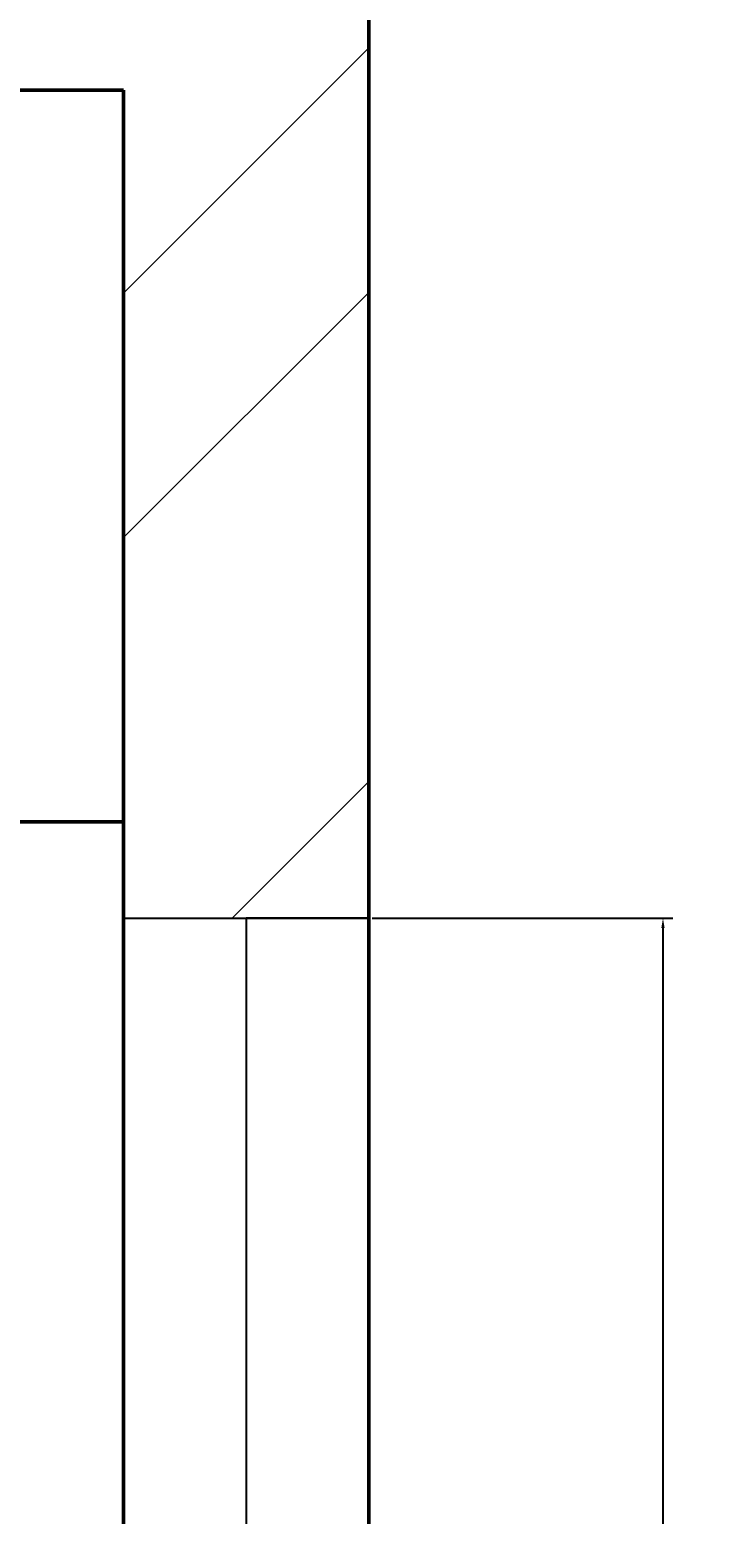
# Model space of a CAD drawing. Units: inches. Extents: x 1901 to 2863, y 888 to 2433.
# Tile 89 of 91: x 2747 to 2759, y 2052 to 2080. Entities that reach past the tile are written whole.
import ezdxf

# ---------------------------------------------------------------- set-up
doc = ezdxf.new("R2010")
doc.units = ezdxf.units.IN
for name, color, linetype, lineweight in [('A-ANNO-DIMS', 2, 'Continuous', 18), ('A-GLAZ', 3, 'Continuous', 25), ('A-WALL', 7, 'Continuous', 50), ('A-WALL-PATT', 8, 'Continuous', 13)]:
    doc.layers.add(name, color=color, linetype=linetype, lineweight=lineweight)
doc.styles.get("Standard").update_dxf_attribs({"font": 'arial.ttf'})
doc.dimstyles.get("Standard").update_dxf_attribs({"dimtxt": 0.18, "dimasz": 0.18, "dimexe": 0.18, "dimexo": 0.0625, "dimgap": 0.09, "dimtad": 0, "dimtih": 1, "dimtoh": 1, "dimdec": 4, "dimzin": 0, "dimdsep": 46, "dimtxsty": 'Standard', "dimcen": 0.09, "dimadec": 0, "dimazin": 0, "dimtfac": 1, "dimtdec": 4, "dimtofl": 0, "dimtmove": 0, "dimatfit": 3, "dimfxl": 1, "dimtolj": 1, "dimtzin": 0, "dimarcsym": 0})

# ---------------------------------------------------------------- blocks, each defined once
blk = doc.blocks.new('WIN-36-5')
for p, q in [((0, 36), (4.5, 36)), ((4.5, 36), (2.25, 36)), ((2.25, 36), (2.25, 0))]:
    blk.add_line(p, q)
blk = doc.blocks.new('*D29')
at = {"layer": 'A-ANNO-DIMS', "color": 0, "lineweight": -2, "transparency": 16777216}
for p, q in [((2752.989, 2063.429), (2758.506, 2063.429)), ((2758.326, 2063.249), (2758.326, 2045.612)), ((2758.326, 2027.609), (2758.326, 2045.245)), ((2752.989, 2027.429), (2758.506, 2027.429))]:
    blk.add_line(p, q, dxfattribs=at)
at = {"layer": 'A-ANNO-DIMS', "color": 0, "transparency": 16777216}
for points in [[(2758.296, 2063.249), (2758.356, 2063.249), (2758.326, 2063.429)], [(2758.296, 2027.609), (2758.356, 2027.609), (2758.326, 2027.429)]]:
    blk.add_solid(points, dxfattribs=at)
at = {"layer": 'Defpoints', "color": 0, "transparency": 16777216}
for p in [(2752.926, 2063.429), (2758.326, 2063.429), (2752.926, 2027.429)]:
    blk.add_point(p, dxfattribs=at)
at = {"layer": 'A-ANNO-DIMS', "color": 0, "transparency": 16777216, "insert": (2758.326, 2045.429), "char_height": 0.18, "attachment_point": 5}
blk.add_mtext('\\A1;WINDOW W6 36 TYP.', dxfattribs=at)

msp = doc.modelspace()

# ---------------------------------------------------------------- hatches: boundary and pattern name
at = {"layer": 'A-WALL-PATT'}
h = msp.add_hatch(dxfattribs=at)
h.set_pattern_fill('ANSI32', color=256)
h.paths.add_polyline_path([(2192.501, 2274.134), (2141.264, 2274.134), (2141.264, 2269.634), (2192.501, 2269.634)])
h.paths.add_polyline_path([(2259.926, 2274.134), (2216.501, 2274.134), (2216.501, 2269.634), (2255.426, 2269.634), (2255.426, 2214.634), (2250.809, 2214.634), (2250.809, 2210.134), (2259.926, 2210.134), (2259.926, 2215.134), (2271.756, 2215.134), (2271.756, 2217.384), (2271.756, 2219.634), (2259.926, 2219.634)])
h.paths.add_polyline_path([(2171.426, 2269.634), (2166.926, 2269.634), (2166.926, 2219.634), (2121.238, 2219.634), (2121.238, 2215.134), (2166.926, 2215.134), (2166.926, 2083.134), (2161.807, 2083.134), (2161.807, 2078.634), (2171.426, 2078.634), (2176.996, 2078.634), (2176.996, 2080.884), (2176.996, 2083.134), (2171.426, 2083.134), (2171.426, 2210.134), (2230.912, 2210.134), (2230.912, 2212.384), (2230.912, 2214.634), (2171.426, 2214.634)])
h.paths.add_polyline_path([(2117.264, 2274.134), (2089.426, 2274.134), (2089.426, 2219.634), (2081.136, 2219.634), (2081.136, 2215.134), (2089.426, 2215.134), (2098.004, 2215.134), (2098.004, 2217.384), (2098.004, 2219.634), (2093.926, 2219.634), (2093.926, 2269.634), (2117.264, 2269.634), (2117.264, 2271.884)])
h.paths.add_polyline_path([(2343.426, 2219.634), (2329.295, 2219.634), (2329.295, 2215.134), (2338.926, 2215.134), (2338.926, 2184.739), (2343.426, 2184.739)])
h.paths.add_polyline_path([(2338.926, 2083.134), (2329.295, 2083.134), (2208.966, 2083.134), (2208.966, 2078.634), (2338.926, 2078.634)])
h.paths.add_polyline_path([(2343.426, 2136.739), (2338.926, 2136.739), (2338.926, 1872.634), (2343.426, 1872.634)])
h.paths.add_polyline_path([(2343.426, 1863.634), (2397.68, 1863.634), (2397.68, 1821.634), (2384.138, 1821.634), (2384.138, 1812.634), (2418.33, 1812.634), (2418.33, 1817.134), (2418.33, 1821.634), (2406.68, 1821.634), (2406.68, 1863.634), (2459.499, 1863.634), (2459.499, 1821.634), (2447.138, 1821.634), (2447.138, 1812.634), (2459.499, 1812.634), (2468.499, 1812.634), (2468.499, 1872.634), (2394.426, 1872.634), (2334.426, 1872.634), (2334.426, 1812.634), (2343.426, 1812.634), (2353.251, 1812.634), (2353.251, 1821.634), (2343.426, 1821.634)])
h.paths.add_polyline_path([(2510.014, 1872.634), (2468.499, 1872.634), (2468.499, 1868.134), (2510.014, 1868.134)])
h.paths.add_polyline_path([(2514.009, 1817.134), (2468.499, 1817.134), (2468.499, 1812.634), (2482.114, 1812.634), (2482.114, 1800.606), (2486.614, 1800.606), (2486.614, 1812.634), (2514.009, 1812.634)])
h.paths.add_polyline_path([(2299.247, 1814.884), (2299.247, 1817.134), (2295.926, 1817.134), (2295.926, 1854.169), (2293.676, 1854.169), (2291.426, 1854.169), (2291.426, 1817.134), (2266.109, 1817.134), (2266.109, 1812.634), (2299.247, 1812.634)])
h.paths.add_polyline_path([(2218.109, 1817.134), (2206.46, 1817.134), (2171.426, 1817.134), (2171.426, 1949.134), (2190.1, 1949.134), (2190.1, 1953.634), (2163.468, 1953.634), (2163.468, 1949.134), (2166.926, 1949.134), (2166.926, 1817.134), (2114.297, 1817.134), (2114.297, 1812.634), (2218.109, 1812.634)])
h.paths.add_polyline_path([(2029.426, 1970.922), (2024.926, 1970.922), (2024.926, 1912.717), (2029.426, 1912.717)])
h.paths.add_polyline_path([(2132.297, 1953.634), (2113.926, 1953.634), (2113.926, 1975.888), (2111.676, 1975.888), (2109.426, 1975.888), (2109.426, 1953.634), (2029.426, 1953.634), (2029.426, 1949.134), (2132.297, 1949.134)])
h.paths.add_polyline_path([(2029.426, 1853.606), (2029.31, 1853.606), (2029.31, 1853.606), (2029.426, 1853.606), (2029.426, 1864.717), (2024.926, 1864.717), (2024.926, 1812.634), (2066.297, 1812.634), (2066.297, 1814.884), (2066.297, 1817.134), (2029.426, 1817.134)])
h.paths.add_polyline_path([(2122.926, 2010.088), (2120.676, 2010.088), (2118.426, 2010.088), (2118.426, 2006.134), (2029.426, 2006.134), (2029.426, 2001.634), (2109.426, 2001.634), (2109.426, 1998.041), (2113.926, 1998.041), (2113.926, 2001.634), (2122.926, 2001.634)])
h.paths.add_polyline_path([(2029.426, 2031.376), (2024.926, 2031.376), (2024.926, 1994.922), (2027.176, 1994.922), (2029.426, 1994.922)])
h.paths.add_polyline_path([(2029.426, 2136.739), (2024.926, 2136.739), (2024.926, 2067.376), (2027.176, 2067.376), (2029.426, 2067.376)])
h.paths.add_polyline_path([(2125.618, 2083.134), (2029.426, 2083.134), (2029.426, 2078.634), (2118.426, 2078.634), (2118.426, 2030.715), (2122.926, 2030.715), (2122.926, 2078.634), (2125.618, 2078.634)])
h.paths.add_polyline_path([(2029.426, 2215.134), (2040.468, 2215.134), (2040.468, 2217.384), (2040.468, 2219.634), (2024.926, 2219.634), (2024.926, 2184.739), (2029.426, 2184.739), (2029.426, 2187.778)])
h.paths.add_polyline_path([(2686.426, 2274.134), (2659.284, 2274.134), (2659.284, 2269.634), (2681.926, 2269.634), (2681.926, 2219.634), (2676.816, 2219.634), (2676.816, 2215.134), (2681.926, 2215.134), (2697.011, 2215.134), (2697.011, 2217.384), (2697.011, 2219.634), (2686.426, 2219.634)])
h.paths.add_polyline_path([(2609.926, 2269.634), (2635.284, 2269.634), (2635.284, 2274.134), (2571.431, 2274.134), (2571.431, 2269.634), (2605.426, 2269.634), (2605.426, 2214.634), (2549.098, 2214.634), (2549.098, 2210.134), (2605.426, 2210.134), (2605.426, 2083.134), (2601.014, 2083.134), (2601.014, 2080.884), (2601.014, 2078.634), (2609.926, 2078.634), (2616.162, 2078.634), (2616.162, 2080.884), (2616.162, 2083.134), (2609.926, 2083.134), (2609.926, 2215.134), (2651.465, 2215.134), (2651.465, 2217.384), (2651.465, 2219.634), (2609.926, 2219.634)])
h.paths.add_polyline_path([(2521.426, 2269.634), (2547.431, 2269.634), (2547.431, 2271.884), (2547.431, 2274.134), (2516.926, 2274.134), (2516.926, 2219.634), (2506.41, 2219.634), (2506.41, 2215.134), (2516.926, 2215.134), (2516.926, 2210.134), (2525.402, 2210.134), (2525.402, 2212.384), (2525.402, 2214.634), (2521.426, 2214.634)])
h.paths.add_polyline_path([(2456.011, 2219.634), (2439.426, 2219.634), (2439.426, 2187.888), (2443.926, 2187.888), (2443.926, 2215.134), (2456.011, 2215.134)])
h.paths.add_polyline_path([(2752.926, 2219.634), (2739.485, 2219.634), (2739.485, 2215.134), (2748.426, 2215.134), (2748.426, 2187.888), (2752.926, 2187.888)])
h.paths.add_polyline_path([(2752.926, 2139.888), (2748.426, 2139.888), (2748.426, 2083.134), (2648.416, 2083.134), (2648.416, 2078.634), (2654.926, 2078.634), (2654.926, 2039.437), (2659.426, 2039.437), (2659.426, 2078.634), (2748.426, 2078.634), (2748.426, 2063.429), (2752.926, 2063.429)])
h.paths.add_polyline_path([(2752.926, 2010.634), (2659.426, 2010.634), (2659.426, 2015.652), (2654.926, 2015.652), (2654.926, 2010.634), (2605.426, 2010.634), (2605.426, 1920.967), (2609.926, 1920.967), (2609.926, 2006.134), (2748.426, 2006.134), (2748.426, 1982.466), (2752.926, 1982.466)])
h.paths.add_polyline_path([(2752.926, 2027.429), (2748.426, 2027.429), (2748.426, 2010.634), (2752.926, 2010.634)])
h.paths.add_polyline_path([(2748.426, 1886.134), (2609.926, 1886.134), (2609.926, 1889.719), (2605.426, 1889.719), (2605.426, 1861.262), (2609.926, 1861.262), (2609.926, 1881.634), (2748.426, 1881.634)])
h.paths.add_polyline_path([(2456.855, 2228.831), (2498.401, 2228.831), (2498.401, 2247.488), (2456.855, 2247.488)], flags=9)
h.paths.add_polyline_path([(2038.602, 2237.418), (2080.174, 2237.418), (2080.174, 2256.075), (2038.602, 2256.075)], flags=9)
h.paths.add_polyline_path([(2292.009, 1062.394), (2539.932, 1062.394), (2539.932, 1099.487), (2292.009, 1099.487)], flags=9)
h.paths.add_polyline_path([(2424.91, 1832.253), (2448.513, 1832.253), (2448.513, 1846.678), (2424.91, 1846.678)], flags=25)
h.paths.add_polyline_path([(2359.076, 1832.253), (2382.678, 1832.253), (2382.678, 1846.678), (2359.076, 1846.678)], flags=25)
h.paths.add_polyline_path([(2352.899, 1684.802), (2367.543, 1684.802), (2367.543, 1697.167), (2352.899, 1697.167)], flags=9)
h.paths.add_polyline_path([(2079.288, 1755.826), (2169.024, 1755.826), (2169.024, 1774.372), (2079.288, 1774.372)], flags=9)
h.paths.add_polyline_path([(2404.09, 1373.857), (2404.09, 1463.593), (2385.544, 1463.593), (2385.544, 1373.857)], flags=9)
h.paths.add_polyline_path([(2268.091, 2236.371), (2309.636, 2236.371), (2309.636, 2255.028), (2268.091, 2255.028)], flags=9)
h.paths.add_polyline_path([(2575.96, 1700.951), (2665.696, 1700.951), (2665.696, 1719.498), (2575.96, 1719.498)], flags=9)
h.paths.add_polyline_path([(2302.962, 1878.474), (2329.524, 1878.474), (2329.524, 1888.777), (2302.962, 1888.777)], flags=9)
h.paths.add_polyline_path([(2097.415, 2240.576), (2126.573, 2240.576), (2126.573, 2259.233), (2097.415, 2259.233)], flags=9)
h.paths.add_polyline_path([(2208.725, 2246.124), (2237.882, 2246.124), (2237.882, 2264.781), (2208.725, 2264.781)], flags=9)
h.paths.add_polyline_path([(2038.147, 1925.958), (2076.987, 1925.958), (2076.987, 1944.615), (2038.147, 1944.615)], flags=9)
h.paths.add_polyline_path([(2239.144, 1926.672), (2288.465, 1926.672), (2288.465, 1945.329), (2239.144, 1945.329)], flags=9)
h.paths.add_polyline_path([(2175.429, 2007.33), (2212.356, 2007.33), (2212.356, 2025.987), (2175.429, 2025.987)], flags=9)
h.paths.add_polyline_path([(2225.034, 2091.794), (2263.875, 2091.794), (2263.875, 2110.451), (2225.034, 2110.451)], flags=9)
h.paths.add_polyline_path([(2035.398, 2098.478), (2074.238, 2098.478), (2074.238, 2117.135), (2035.398, 2117.135)], flags=9)
h.paths.add_polyline_path([(2050.102, 2029.209), (2083.26, 2029.209), (2083.26, 2047.866), (2050.102, 2047.866)], flags=9)
h.paths.add_polyline_path([(2069.677, 1956.719), (2098.835, 1956.719), (2098.835, 1975.376), (2069.677, 1975.376)], flags=25)
h.paths.add_polyline_path([(2328.62, 1753.336), (2361.663, 1753.336), (2361.663, 1771.993), (2328.62, 1771.993)], flags=9)
h.paths.add_polyline_path([(2395.162, 2060.888), (2395.162, 2140.654), (2378.676, 2140.654), (2378.676, 2060.888)], flags=9)
h.paths.add_polyline_path([(2463.728, 2059.02), (2492.886, 2059.02), (2492.886, 2077.677), (2463.728, 2077.677)], flags=9)
h.paths.add_polyline_path([(2458.027, 2181.536), (2496.868, 2181.536), (2496.868, 2200.194), (2458.027, 2200.194)], flags=9)
h.paths.add_polyline_path([(2527.577, 2243.074), (2556.735, 2243.074), (2556.735, 2261.731), (2527.577, 2261.731)], flags=9)
h.paths.add_polyline_path([(2694.461, 2232.767), (2736.033, 2232.767), (2736.033, 2251.425), (2694.461, 2251.425)], flags=9)
h.paths.add_polyline_path([(2637.821, 2249.225), (2666.979, 2249.225), (2666.979, 2267.882), (2637.821, 2267.882)], flags=9)
h.paths.add_polyline_path([(2623.687, 2183.541), (2662.528, 2183.541), (2662.528, 2202.199), (2623.687, 2202.199)], flags=9)
h.paths.add_polyline_path([(2691.965, 2021.5), (2725.124, 2021.5), (2725.124, 2040.157), (2691.965, 2040.157)], flags=9)
h.paths.add_polyline_path([(2621.043, 1975.912), (2662.335, 1975.912), (2662.335, 1994.569), (2621.043, 1994.569)], flags=25)
h.paths.add_polyline_path([(2479.032, 1927.62), (2519.844, 1927.62), (2519.844, 1946.277), (2479.032, 1946.277)], flags=9)
h.paths.add_polyline_path([(2670.941, 1849.076), (2716.005, 1849.076), (2716.005, 1867.734), (2670.941, 1867.734)], flags=9)
h.paths.add_polyline_path([(2523.613, 1782.956), (2550.175, 1782.956), (2550.175, 1793.26), (2523.613, 1793.26)], flags=9)
h.paths.add_polyline_path([(2450.841, 1207.331), (2492.386, 1207.331), (2492.386, 1225.989), (2450.841, 1225.989)], flags=9)
h.paths.add_polyline_path([(2527.751, 1203.841), (2556.908, 1203.841), (2556.908, 1222.499), (2527.751, 1222.499)], flags=9)
h.paths.add_polyline_path([(2639.111, 1207.2), (2668.268, 1207.2), (2668.268, 1225.857), (2639.111, 1225.857)], flags=9)
h.paths.add_polyline_path([(2692.594, 1218.965), (2734.167, 1218.965), (2734.167, 1237.623), (2692.594, 1237.623)], flags=9)
h.paths.add_polyline_path([(2669.266, 1366.329), (2708.106, 1366.329), (2708.106, 1384.987), (2669.266, 1384.987)], flags=9)
h.paths.add_polyline_path([(2463.313, 1358.031), (2502.153, 1358.031), (2502.153, 1376.688), (2463.313, 1376.688)], flags=9)
h.paths.add_polyline_path([(2494.725, 1449.963), (2531.652, 1449.963), (2531.652, 1468.62), (2494.725, 1468.62)], flags=9)
h.paths.add_polyline_path([(2675.565, 1422.157), (2708.724, 1422.157), (2708.724, 1440.815), (2675.565, 1440.815)], flags=9)
h.paths.add_polyline_path([(2685.634, 1493.891), (2714.792, 1493.891), (2714.792, 1512.548), (2685.634, 1512.548)], flags=9)
h.paths.add_polyline_path([(2686.805, 1529.913), (2725.645, 1529.913), (2725.645, 1548.57), (2686.805, 1548.57)], flags=9)
h.paths.add_polyline_path([(2503.651, 1537.991), (2552.972, 1537.991), (2552.972, 1556.648), (2503.651, 1556.648)], flags=9)
h.paths.add_polyline_path([(2291.713, 1643.504), (2318.275, 1643.504), (2318.275, 1653.807), (2291.713, 1653.807)], flags=9)
h.paths.add_polyline_path([(2450.626, 1610.52), (2477.189, 1610.52), (2477.189, 1620.824), (2450.626, 1620.824)], flags=9)
h.paths.add_polyline_path([(2359.985, 1551.814), (2422.253, 1551.814), (2422.253, 1562.117), (2359.985, 1562.117)], flags=9)
h.paths.add_polyline_path([(2280.106, 1249.006), (2321.651, 1249.006), (2321.651, 1267.663), (2280.106, 1267.663)], flags=9)
h.paths.add_polyline_path([(2164.057, 1274.232), (2193.215, 1274.232), (2193.215, 1292.889), (2164.057, 1292.889)], flags=9)
h.paths.add_polyline_path([(2118.21, 1277.694), (2151.252, 1277.694), (2151.252, 1296.351), (2118.21, 1296.351)], flags=9)
h.paths.add_polyline_path([(2031.946, 1268.529), (2073.519, 1268.529), (2073.519, 1287.187), (2031.946, 1287.187)], flags=9)
h.paths.add_polyline_path([(2050.199, 1409.079), (2089.04, 1409.079), (2089.04, 1427.736), (2050.199, 1427.736)], flags=9)
h.paths.add_polyline_path([(2243.743, 1421.032), (2282.584, 1421.032), (2282.584, 1439.689), (2243.743, 1439.689)], flags=9)
h.paths.add_polyline_path([(2190.746, 1509.769), (2231.558, 1509.769), (2231.558, 1528.426), (2190.746, 1528.426)], flags=9)
h.paths.add_polyline_path([(2058.392, 1475.415), (2091.55, 1475.415), (2091.55, 1494.073), (2058.392, 1494.073)], flags=9)
h.paths.add_polyline_path([(2062.447, 1553.09), (2091.605, 1553.09), (2091.605, 1571.747), (2062.447, 1571.747)], flags=9)
h.paths.add_polyline_path([(2219.524, 1590.365), (2266.147, 1590.365), (2266.147, 1609.022), (2219.524, 1609.022)], flags=9)
h.paths.add_polyline_path([(2041.072, 1584.188), (2079.912, 1584.188), (2079.912, 1602.845), (2041.072, 1602.845)], flags=9)

# ---------------------------------------------------------------- linework, layer by layer
at = {"layer": 'A-WALL'}
for p, q in [((2752.926, 2219.634), (2752.926, 1812.634)), ((2659.426, 2078.634), (2748.426, 2078.634)), ((2748.426, 2078.634), (2748.426, 2010.634)), ((2734.984, 2065.199), (2748.426, 2065.199))]:
    msp.add_line(p, q, dxfattribs=at)

# ---------------------------------------------------------------- block references
at = {"layer": 'A-GLAZ'}
msp.add_blockref('WIN-36-5', (2748.426, 2027.429), dxfattribs=at)

# ---------------------------------------------------------------- dimensions: what is measured, and where the dimension line sits
at = {"layer": 'A-ANNO-DIMS'}
dim = msp.add_linear_dim(base=(2758.326, 2063.429), p1=(2752.926, 2027.429), p2=(2752.926, 2063.429), angle=90, text='WINDOW W6 <> TYP.', dimstyle='Standard', override={"dimdec": 0, "dimlfac": 1, "dimrnd": 0, "dimzin": 0, "dimdsep": 46, "dimlunit": 2}, dxfattribs=at)
dim.commit()
dim.dimension.update_dxf_attribs({"geometry": '*D29', "text_midpoint": (2758.326, 2045.429)})

doc.saveas('drawing.dxf')
